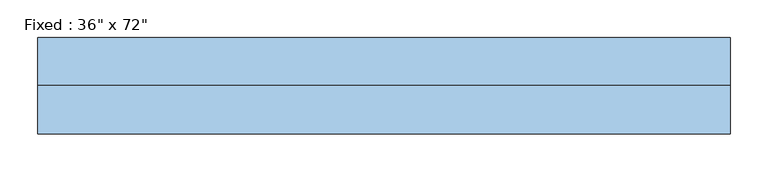
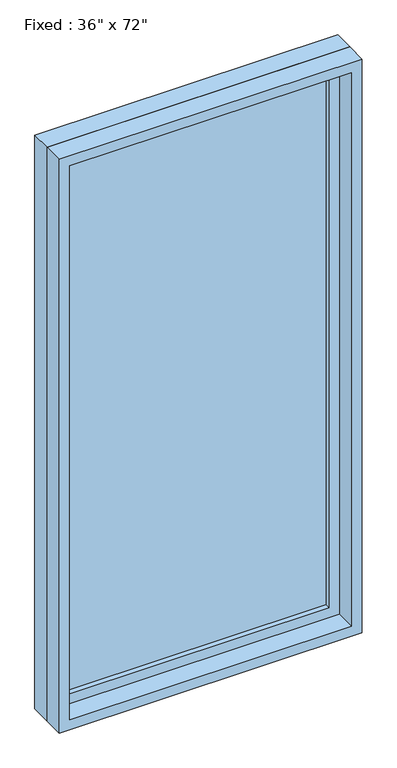
"""IFC4 building model written with IfcOpenShell, lengths in millimetres: window geometry."""

from ifc_helpers import new_model, si_unit, frame, origin, place, context, project, spatial, polyline, outline, extrude, source, transform, mapped, element, save


def window_7da3115e(model_context):
    return source(origin(), model_context, "Body", "SweptSolid", [
        extrude(outline(polyline([(355.6, 15.875), (-431.8, 15.875), (-431.8, 28.575), (355.6, 28.575), (355.6, 15.875)])), frame((0.0, 0.0, 368.3), z_axis=(0.0, 0.0, 1.0), x_axis=(1.0, 0.0, 0.0)), (0.0, 0.0, 1.0), 1701.8),
        extrude(outline(polyline([(2114.55, -476.25), (323.85, -476.25), (323.85, 400.05), (2114.55, 400.05), (2114.55, -476.25)]), holes=[polyline([(2070.1, -431.8), (2070.1, 355.6), (368.3, 355.6), (368.3, -431.8), (2070.1, -431.8)])]), frame((0.0, 0.0, 0.0), z_axis=(0.0, 1.0, 0.0), x_axis=(0.0, 0.0, 1.0)), (0.0, 0.0, 1.0), 44.45),
        extrude(outline(polyline([(2133.6, -495.3), (304.8, -495.3), (304.8, 419.1), (2133.6, 419.1), (2133.6, -495.3)]), holes=[polyline([(2101.85, -463.55), (2101.85, 387.35), (336.55, 387.35), (336.55, -463.55), (2101.85, -463.55)])]), frame((0.0, -63.5, 0.0), z_axis=(0.0, 1.0, 0.0), x_axis=(0.0, 0.0, 1.0)), (0.0, 0.0, 1.0), 63.5),
        extrude(outline(polyline([(2133.6, 419.1), (2133.6, -495.3), (304.8, -495.3), (304.8, 419.1), (2133.6, 419.1)]), holes=[polyline([(2114.55, 400.05), (323.85, 400.05), (323.85, -476.25), (2114.55, -476.25), (2114.55, 400.05)])]), frame((0.0, 0.0, 0.0), z_axis=(0.0, 1.0, 0.0), x_axis=(0.0, 0.0, 1.0)), (0.0, 0.0, 1.0), 63.5),
    ])


if __name__ == "__main__":
    model = new_model("IFC4")
    model_context = context("Model", 3, world=origin())
    ifc_project = project(units=[si_unit("LENGTHUNIT", "METRE", prefix="MILLI")], contexts=[model_context])
    site = spatial("IfcSite", under=ifc_project)
    building = spatial("IfcBuilding", under=site)
    placement = place(None, origin())
    window_shape = window_7da3115e(model_context)
    element("IfcWindow", 1, ObjectType="Fixed : 36\" x 72\"", at=placement, inside=building, context=model_context, shape_type="MappedRepresentation", body=[
        mapped(window_shape, transform((0.0, 0.0, 0.0), x_axis=(1.0, 0.0, 0.0), y_axis=(0.0, 1.0, 0.0), z_axis=(0.0, 0.0, 1.0))),
    ])
    save(model, "model.ifc")

# Revit data of these elements
# Type "Fixed : 36\" x 72\""
#   Type Mark = "9"
#   Assembly Code = "B2020100"
#   Height = 6' - 0"
#   Default Sill Height = 1' - 0"
#   Width = 3' - 0"
#   Window Inset = 0' - 0 3/4"
#   Glass Pane Material = Glass
#   Sash Material = Sash
#   Wall Closure = (empty or 0)
# Element 1 (IfcWindow, "Fixed : 36\" x 72\"")
#   Materials on its faces: "Sash", "Glass"
# Materials
#   "Glass": class "Glass", colour RGB 218 227 224, transparency 0.85, Description = "Soda Lime Glass", Cost = 0
#   "Sash": class "Wood", colour RGB 136 99 55, transparency 0
